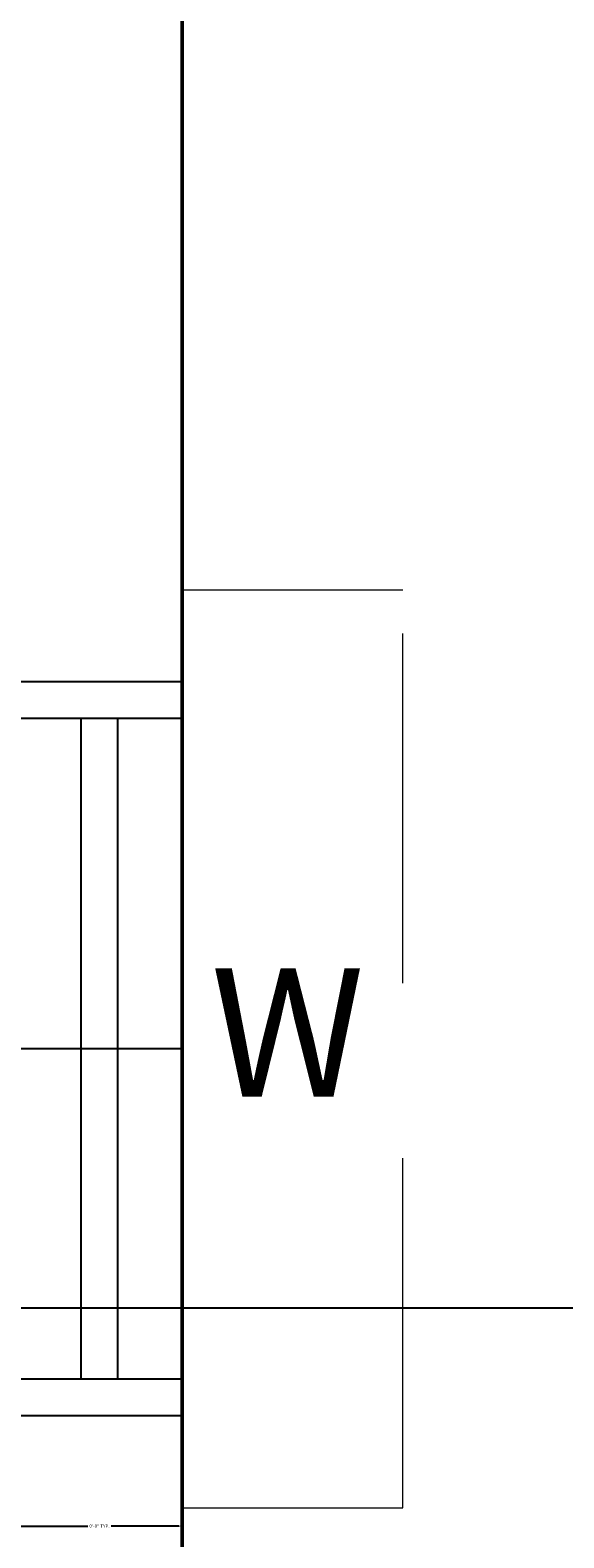
# Model space of a CAD drawing. Units: inches. Extents: x 37 to 824, y -700 to 234.
# Tile 66 of 77: x 420 to 449, y -75 to 8. Entities that reach past the tile are written whole.
import ezdxf

# ---------------------------------------------------------------- set-up
doc = ezdxf.new("R2010")
doc.units = ezdxf.units.IN
doc.header["$MEASUREMENT"] = 0
doc.linetypes.add('DASHED', pattern=[19.05, 12.7, -6.35])
for name, color, linetype, lineweight in [('A-ANNO-DIMS', 2, 'Continuous', 18), ('A-ANNO-TEXT', 7, 'Continuous', 18), ('A-GLAZ', 4, 'Continuous', 25), ('A-ROOF-OVHD', 1, 'DASHED', 18), ('A-WALL', 2, 'Continuous', 50)]:
    doc.layers.add(name, color=color, linetype=linetype, lineweight=lineweight)
doc.styles.get("Standard").update_dxf_attribs({"font": 'arial.ttf'})
doc.dimstyles.get("Standard").update_dxf_attribs({"dimtxt": 0.18, "dimasz": 0.18, "dimexe": 0.18, "dimexo": 0.0625, "dimgap": 0.09, "dimtad": 0, "dimtih": 1, "dimtoh": 1, "dimdec": 1, "dimzin": 0, "dimdsep": 46, "dimlunit": 4, "dimtxsty": 'Standard', "dimcen": 0.09, "dimadec": 0, "dimazin": 0, "dimtfac": 1, "dimtdec": 1, "dimtofl": 0, "dimtmove": 0, "dimatfit": 3, "dimfxl": 1, "dimtolj": 1, "dimtzin": 0, "dimarcsym": 0})

# ---------------------------------------------------------------- blocks, each defined once
blk = doc.blocks.new('WIN-900')
for p, q in [((0, 9), (0, 0)), ((2, 9), (2, 0)), ((20, 9), (20, 0)), ((38, 9), (38, 0)), ((40, 9), (40, 0)), ((38, 5.5), (2, 5.5)), ((38, 3.5), (2, 3.5))]:
    blk.add_line(p, q)
blk = doc.blocks.new('*D39')
at = {"layer": 'A-ANNO-DIMS', "color": 0, "lineweight": -2, "ltscale": 0.5, "transparency": 16777216}
for p, q in [((419.077, -67.972), (419.077, -74.09)), ((428.077, -67.972), (428.077, -74.09)), ((419.257, -73.91), (422.939, -73.91)), ((427.897, -73.91), (424.216, -73.91))]:
    blk.add_line(p, q, dxfattribs=at)
at = {"layer": 'A-ANNO-DIMS', "color": 0, "ltscale": 0.5, "transparency": 16777216}
for points in [[(419.257, -73.88), (419.257, -73.94), (419.077, -73.91)], [(427.897, -73.88), (427.897, -73.94), (428.077, -73.91)]]:
    blk.add_solid(points, dxfattribs=at)
at = {"layer": 'Defpoints', "color": 0, "ltscale": 0.5, "transparency": 16777216}
for p in [(419.077, -67.91), (428.077, -67.91), (428.077, -73.91)]:
    blk.add_point(p, dxfattribs=at)
at = {"layer": 'A-ANNO-DIMS', "color": 0, "ltscale": 0.5, "transparency": 16777216, "insert": (423.577, -73.91), "char_height": 0.18, "attachment_point": 5}
blk.add_mtext('\\A1;0\'-9" TYP.', dxfattribs=at)
blk = doc.blocks.new('*D64')
at = {"layer": 'A-ANNO-DIMS', "color": 0, "lineweight": -2, "ltscale": 0.5, "transparency": 16777216}
for p, q in [((428.14, 191.09), (513.773, 191.09)), ((513.593, 190.91), (513.593, -87.228)), ((513.593, -365.73), (513.593, -87.591)), ((428.14, -365.91), (513.773, -365.91))]:
    blk.add_line(p, q, dxfattribs=at)
at = {"layer": 'A-ANNO-DIMS', "color": 0, "ltscale": 0.5, "transparency": 16777216}
for points in [[(513.563, 190.91), (513.623, 190.91), (513.593, 191.09)], [(513.563, -365.73), (513.623, -365.73), (513.593, -365.91)]]:
    blk.add_solid(points, dxfattribs=at)
at = {"layer": 'Defpoints', "color": 0, "ltscale": 0.5, "transparency": 16777216}
for p in [(428.077, 191.09), (428.077, -365.91), (513.593, -365.91)]:
    blk.add_point(p, dxfattribs=at)
at = {"layer": 'A-ANNO-DIMS', "color": 0, "ltscale": 0.5, "transparency": 16777216, "insert": (513.593, -87.41), "char_height": 0.18, "attachment_point": 5}
blk.add_mtext('\\A1;46\'-5"', dxfattribs=at)
blk = doc.blocks.new('*D79')
at = {"layer": 'A-ANNO-DIMS', "color": 0, "lineweight": -2, "ltscale": 0.5, "transparency": 16777216}
for p, q in [((299.14, -62.022), (513.773, -62.022)), ((513.593, -62.202), (513.593, -81.784)), ((513.593, -101.73), (513.593, -82.148)), ((296.14, -101.91), (513.773, -101.91))]:
    blk.add_line(p, q, dxfattribs=at)
at = {"layer": 'A-ANNO-DIMS', "color": 0, "ltscale": 0.5, "transparency": 16777216}
for points in [[(513.563, -62.202), (513.623, -62.202), (513.593, -62.022)], [(513.563, -101.73), (513.623, -101.73), (513.593, -101.91)]]:
    blk.add_solid(points, dxfattribs=at)
at = {"layer": 'Defpoints', "color": 0, "ltscale": 0.5, "transparency": 16777216}
for p in [(299.077, -62.022), (296.077, -101.91), (513.593, -101.91)]:
    blk.add_point(p, dxfattribs=at)
at = {"layer": 'A-ANNO-DIMS', "color": 0, "ltscale": 0.5, "transparency": 16777216, "insert": (513.593, -81.966), "char_height": 0.18, "attachment_point": 5}
blk.add_mtext('\\A1;3\'-4"', dxfattribs=at)

msp = doc.modelspace()

# ---------------------------------------------------------------- linework, layer by layer
at = {"layer": 'A-ROOF-OVHD', "ltscale": 1.5}
for p, q in [((428.077, -27.91), (428.077, -22.91)), ((428.077, -22.91), (440.077, -22.91)), ((440.077, -72.91), (440.077, -22.91)), ((428.077, -67.91), (428.077, -72.91)), ((428.077, -72.91), (440.077, -72.91))]:
    msp.add_line(p, q, dxfattribs=at)
at = {"layer": 'A-WALL'}
for p, q in [((428.077, 75.09), (428.077, 6.09)), ((428.077, 6.09), (428.077, -110.91))]:
    msp.add_line(p, q, dxfattribs=at)

# ---------------------------------------------------------------- block references
at = {"layer": 'A-GLAZ', "rotation": 270.0000000000001}
msp.add_blockref('WIN-900', (419.077, -27.909), dxfattribs=at)

# ---------------------------------------------------------------- texts
at = {"layer": 'A-ANNO-TEXT'}
msp.add_text('W', height=7, dxfattribs=at).set_placement((429.625, -50.521))

# ---------------------------------------------------------------- dimensions: what is measured, and where the dimension line sits
at = {"layer": 'A-ANNO-DIMS', "ltscale": 0.5}
for base, p1, p2, picture, middle in [((513.593, -365.91), (428.077, 191.09), (428.077, -365.91), '*D64', (513.593, -87.41)), ((513.593, -101.91), (299.077, -62.022), (296.077, -101.91), '*D79', (513.593, -81.966))]:
    dim = msp.add_linear_dim(base=base, p1=p1, p2=p2, angle=90, dimstyle='Standard', override={"dimdec": 1, "dimlfac": 1, "dimrnd": 0, "dimzin": 1, "dimdsep": 46, "dimlunit": 4, "dimfrac": 2}, dxfattribs=at)
    dim.commit()
    dim.dimension.update_dxf_attribs({"geometry": picture, "text_midpoint": middle})
dim = msp.add_linear_dim(base=(428.077, -73.91), p1=(419.077, -67.91), p2=(428.077, -67.91), angle=0, text='<> TYP.', dimstyle='Standard', override={"dimdec": 1, "dimlfac": 1, "dimrnd": 0, "dimzin": 1, "dimdsep": 46, "dimlunit": 4, "dimfrac": 2}, dxfattribs=at)
dim.commit()
dim.dimension.update_dxf_attribs({"geometry": '*D39', "text_midpoint": (423.577, -73.91)})

doc.saveas('drawing.dxf')
